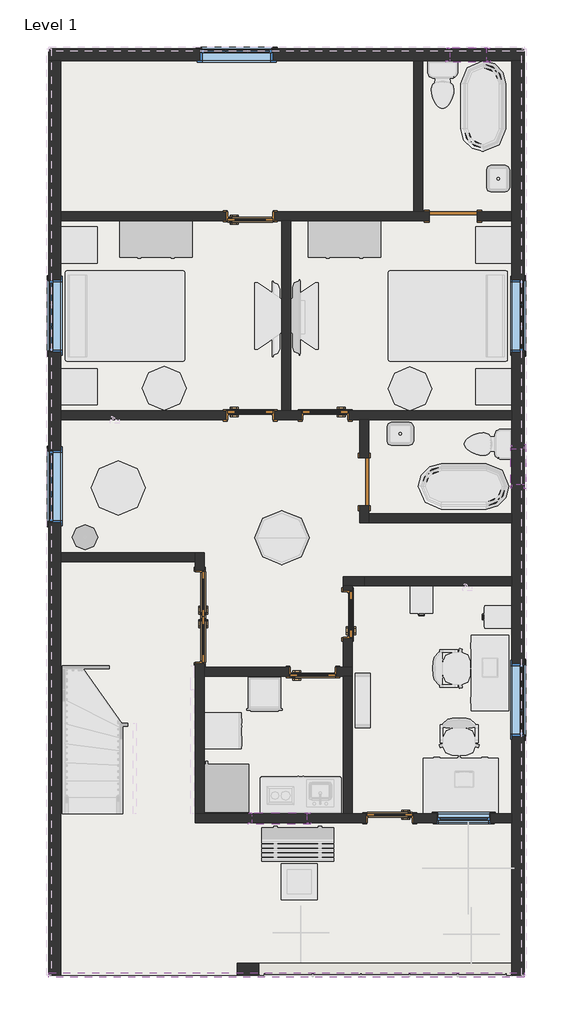
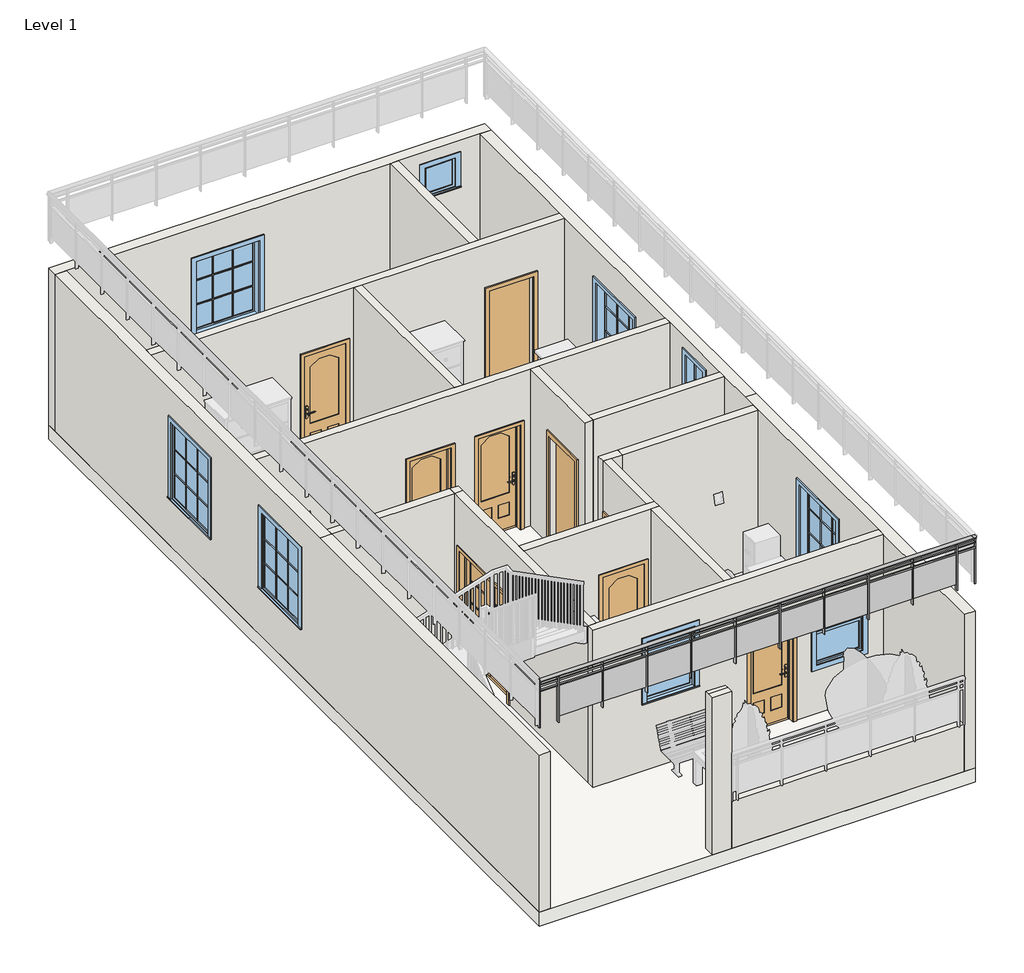
# One storey, part 1 of 4: 19 walls, 9 doors, 9 windows, 1 railing, 1 slab.
"""IFC4 building model written with IfcOpenShell, lengths in millimetres."""

from ifc_helpers import new_model, si_unit, point, frame, origin, origin_with_axes, place, context, project, spatial, polyline, ellipse_curve, trimmed, outline, extrude, faceted_brep, transform, mapped, element, save
from ifc_brep_helpers import plane_surface, extruded_surface, advanced_brep
from components import door_14b9be53, door_4b146b56, door_94998e6c, door_bb092f7c, door_377e7377, window_99fc0ff6, window_d24d93a6, window_e41d21a6

model = new_model("IFC4")

# Units and contexts
model_context = context("Model", 3, world=origin())
ifc_project = project(units=[si_unit("LENGTHUNIT", "METRE", prefix="MILLI")], contexts=[model_context])

# Site, building, storey
site = spatial("IfcSite", under=ifc_project)
building = spatial("IfcBuilding", under=site)
storey = spatial("IfcBuildingStorey", under=building, Name="Level 1", Elevation=0.0)

# Doors
placement = place(None, origin())
door_shape = door_14b9be53(model_context)
element("IfcDoor", 1, ObjectType="30\" x 80\"", at=placement, inside=storey, context=model_context, shape_type="MappedRepresentation", body=[
    mapped(door_shape, transform((-9119.5568901, 3176.746124, 0.0), x_axis=(-1.0, 0.0, 0.0), y_axis=(0.0, -1.0, 0.0), z_axis=(0.0, 0.0, 1.0))),
])
element("IfcDoor", 2, ObjectType="30\" x 80\"", at=placement, inside=storey, context=model_context, shape_type="MappedRepresentation", body=[
    mapped(door_shape, transform((-8532.1818901, 4145.121124, 0.0), x_axis=(0.0, -1.0, 0.0), y_axis=(1.0, 0.0, 0.0), z_axis=(0.0, 0.0, 1.0))),
])
element("IfcDoor", 3, ObjectType="30\" x 80\"", at=placement, inside=storey, context=model_context, shape_type="MappedRepresentation", body=[
    mapped(door_shape, transform((-8910.0068901, 7501.096124, 0.0), x_axis=(1.0, 0.0, 0.0), y_axis=(0.0, 1.0, 0.0), z_axis=(0.0, 0.0, 1.0))),
])
element("IfcDoor", 4, ObjectType="30\" x 80\"", at=placement, inside=storey, context=model_context, shape_type="MappedRepresentation", body=[
    mapped(door_shape, transform((-10173.6568901, 10847.546124, 0.0), x_axis=(-1.0, 0.0, 0.0), y_axis=(0.0, -1.0, 0.0), z_axis=(0.0, 0.0, 1.0))),
])
element("IfcDoor", 5, ObjectType="30\" x 80\"", at=placement, inside=storey, context=model_context, shape_type="MappedRepresentation", body=[
    mapped(door_shape, transform((-7824.1568901, 719.296124, 0.0), x_axis=(1.0, 0.0, 0.0), y_axis=(0.0, 1.0, 0.0), z_axis=(0.0, 0.0, 1.0))),
])
door_2_shape = door_4b146b56(model_context)
element("IfcDoor", 6, ObjectType="30\" x 80\"", at=placement, inside=storey, context=model_context, shape_type="MappedRepresentation", body=[
    mapped(door_2_shape, transform((-10173.6568901, 7501.096124, 0.0), x_axis=(-1.0, 0.0, 0.0), y_axis=(0.0, -1.0, 0.0), z_axis=(0.0, 0.0, 1.0))),
])
door_3_shape = door_94998e6c(model_context)
element("IfcDoor", 7, ObjectType="Door-Exterior-Double-Full Glass-Wood_Clad : 60\" x 80\"", at=placement, inside=storey, context=model_context, shape_type="MappedRepresentation", body=[
    mapped(door_3_shape, transform((-11021.3818901, 4107.021124, 0.0), x_axis=(0.0, -1.0, 0.0), y_axis=(1.0, 0.0, 0.0), z_axis=(0.0, 0.0, 1.0))),
])
door_4_shape = door_bb092f7c(model_context)
element("IfcDoor", 8, ObjectType="Single-Flush : 32\" x 84\"", at=placement, inside=storey, context=model_context, shape_type="MappedRepresentation", body=[
    mapped(door_4_shape, transform((-6757.3568901, 10850.721124, 0.0), x_axis=(-1.0, 0.0, 0.0), y_axis=(0.0, -1.0, 0.0), z_axis=(0.0, 0.0, 1.0))),
])
door_5_shape = door_377e7377(model_context)
element("IfcDoor", 9, ObjectType="Single-Flush : 32\" x 84\"", at=placement, inside=storey, context=model_context, shape_type="MappedRepresentation", body=[
    mapped(door_5_shape, transform((-8255.9568901, 6380.321124, 0.0), x_axis=(0.0, -1.0, 0.0), y_axis=(1.0, 0.0, 0.0), z_axis=(0.0, 0.0, 1.0))),
])

# Railing
element("IfcRailing", 10, ObjectType="Glass Panel - Bottom Fill", at=placement, inside=storey, context=model_context, shape_type="SolidModel", body=[
    advanced_brep(
    [(-13564.5568901, -1887.378876, 4495.8), (-13564.5568901, -1963.578876, 4495.8), (-5563.5568901, -1887.378876, 4495.8), (-5563.5568901, -1963.578876, 4495.8)],
    [
        (0, 1, ellipse_curve(frame((-13564.5568901, -1925.478876, 4495.8), z_axis=(-1.0, 0.0, 0.0), x_axis=(0.0, -1.0, 0.0)), 38.1, 28.575)),
        (1, 0, ellipse_curve(frame((-13564.5568901, -1925.478876, 4495.8), z_axis=(-1.0, 0.0, 0.0), x_axis=(0.0, -1.0, 0.0)), 38.1, 28.575)),
        (2, 3, ellipse_curve(frame((-5563.5568901, -1925.478876, 4495.8), z_axis=(1.0, 0.0, 0.0), x_axis=(0.0, -1.0, 0.0)), 38.1, 28.575)),
        (3, 2, ellipse_curve(frame((-5563.5568901, -1925.478876, 4495.8), z_axis=(1.0, 0.0, 0.0), x_axis=(0.0, -1.0, 0.0)), 38.1, 28.575)),
        (0, 2),
        (3, 1),
    ],
    [
        plane_surface(frame((-13564.5568901, -1925.478876, 4495.8), z_axis=(-1.0, 0.0, 0.0), x_axis=(0.0, 1.0, 0.0))),
        plane_surface(frame((-5563.5568901, -1925.478876, 4495.8), z_axis=(1.0, 0.0, 0.0), x_axis=(0.0, 1.0, 0.0))),
        extruded_surface(trimmed(ellipse_curve(frame((-5563.5568901, -1925.478876, 4495.8), z_axis=(-1.0, 0.0, 0.0), x_axis=(0.0, -1.0, 0.0)), 38.1, 28.575), [point((-5563.5568901, -1887.378876, 4495.8))], [point((-5563.5568901, -1963.578876, 4495.8))], True, "CARTESIAN"), (-8001.000000000001, 0.0, 0.0), 8001.000000000001),
        extruded_surface(trimmed(ellipse_curve(frame((-5563.5568901, -1925.478876, 4495.8), z_axis=(-1.0, 0.0, 0.0), x_axis=(0.0, -1.0, 0.0)), 38.1, 28.575), [point((-5563.5568901, -1963.578876, 4495.8))], [point((-5563.5568901, -1887.378876, 4495.8))], True, "CARTESIAN"), (-8001.000000000001, 0.0, 0.0), 8001.000000000001),
    ],
    [
        (0, [[1, 2]]),
        (1, [[3, 4]]),
        (2, [[-1, 5, -4, 6]]),
        (3, [[-2, -6, -3, -5]]),
    ],
),
    extrude(outline(polyline([(-13564.5568901, -1938.178876), (-13564.5568901, -1912.778876), (-5563.5568901, -1912.778876), (-5563.5568901, -1938.178876), (-13564.5568901, -1938.178876)])), frame((0.0, 0.0, 4381.5), z_axis=(0.0, 0.0, 1.0), x_axis=(1.0, 0.0, 0.0)), (0.0, 0.0, 1.0), 25.4),
    extrude(outline(polyline([(-13564.5568901, -1938.178876), (-13564.5568901, -1912.778876), (-5563.5568901, -1912.778876), (-5563.5568901, -1938.178876), (-13564.5568901, -1938.178876)])), frame((0.0, 0.0, 4279.9), z_axis=(0.0, 0.0, 1.0), x_axis=(1.0, 0.0, 0.0)), (0.0, 0.0, 1.0), 25.4),
    extrude(outline(polyline([(-5912.8068901, -1950.878876), (-5912.8068901, -1900.078876), (-5900.1068901, -1900.078876), (-5900.1068901, -1950.878876), (-5912.8068901, -1950.878876)])), frame((0.0, 0.0, 3581.4), z_axis=(0.0, 0.0, 1.0), x_axis=(1.0, 0.0, 0.0)), (0.0, 0.0, 1.0), 885.6788223),
    extrude(outline(polyline([(-6719.2568901, -1918.943719), (-5906.4568901, -1918.943719), (-5906.4568901, -1925.293719), (-6719.2568901, -1925.293719), (-6719.2568901, -1918.943719)])), frame((0.0, 0.0, 3683.0), z_axis=(0.0, 0.0, 1.0), x_axis=(1.0, 0.0, 0.0)), (0.0, 0.0, 1.0), 596.9),
    extrude(outline(polyline([(-6725.6068901, -1950.878876), (-6725.6068901, -1900.078876), (-6712.9068901, -1900.078876), (-6712.9068901, -1950.878876), (-6725.6068901, -1950.878876)])), frame((0.0, 0.0, 3581.4), z_axis=(0.0, 0.0, 1.0), x_axis=(1.0, 0.0, 0.0)), (0.0, 0.0, 1.0), 885.6788223),
    extrude(outline(polyline([(-7532.0568901, -1918.943719), (-6719.2568901, -1918.943719), (-6719.2568901, -1925.293719), (-7532.0568901, -1925.293719), (-7532.0568901, -1918.943719)])), frame((0.0, 0.0, 3683.0), z_axis=(0.0, 0.0, 1.0), x_axis=(1.0, 0.0, 0.0)), (0.0, 0.0, 1.0), 596.9),
    extrude(outline(polyline([(-7538.4068901, -1950.878876), (-7538.4068901, -1900.078876), (-7525.7068901, -1900.078876), (-7525.7068901, -1950.878876), (-7538.4068901, -1950.878876)])), frame((0.0, 0.0, 3581.4), z_axis=(0.0, 0.0, 1.0), x_axis=(1.0, 0.0, 0.0)), (0.0, 0.0, 1.0), 885.6788223),
    extrude(outline(polyline([(-8344.8568901, -1918.943719), (-7532.0568901, -1918.943719), (-7532.0568901, -1925.293719), (-8344.8568901, -1925.293719), (-8344.8568901, -1918.943719)])), frame((0.0, 0.0, 3683.0), z_axis=(0.0, 0.0, 1.0), x_axis=(1.0, 0.0, 0.0)), (0.0, 0.0, 1.0), 596.9),
    extrude(outline(polyline([(-8351.2068901, -1950.878876), (-8351.2068901, -1900.078876), (-8338.5068901, -1900.078876), (-8338.5068901, -1950.878876), (-8351.2068901, -1950.878876)])), frame((0.0, 0.0, 3581.4), z_axis=(0.0, 0.0, 1.0), x_axis=(1.0, 0.0, 0.0)), (0.0, 0.0, 1.0), 885.6788223),
    extrude(outline(polyline([(-9157.6568901, -1918.943719), (-8344.8568901, -1918.943719), (-8344.8568901, -1925.293719), (-9157.6568901, -1925.293719), (-9157.6568901, -1918.943719)])), frame((0.0, 0.0, 3683.0), z_axis=(0.0, 0.0, 1.0), x_axis=(1.0, 0.0, 0.0)), (0.0, 0.0, 1.0), 596.9),
    extrude(outline(polyline([(-9164.0068901, -1950.878876), (-9164.0068901, -1900.078876), (-9151.3068901, -1900.078876), (-9151.3068901, -1950.878876), (-9164.0068901, -1950.878876)])), frame((0.0, 0.0, 3581.4), z_axis=(0.0, 0.0, 1.0), x_axis=(1.0, 0.0, 0.0)), (0.0, 0.0, 1.0), 885.6788223),
    extrude(outline(polyline([(-9970.4568901, -1918.943719), (-9157.6568901, -1918.943719), (-9157.6568901, -1925.293719), (-9970.4568901, -1925.293719), (-9970.4568901, -1918.943719)])), frame((0.0, 0.0, 3683.0), z_axis=(0.0, 0.0, 1.0), x_axis=(1.0, 0.0, 0.0)), (0.0, 0.0, 1.0), 596.9),
    extrude(outline(polyline([(-9976.8068901, -1950.878876), (-9976.8068901, -1900.078876), (-9964.1068901, -1900.078876), (-9964.1068901, -1950.878876), (-9976.8068901, -1950.878876)])), frame((0.0, 0.0, 3581.4), z_axis=(0.0, 0.0, 1.0), x_axis=(1.0, 0.0, 0.0)), (0.0, 0.0, 1.0), 885.6788223),
    extrude(outline(polyline([(-10783.2568901, -1918.943719), (-9970.4568901, -1918.943719), (-9970.4568901, -1925.293719), (-10783.2568901, -1925.293719), (-10783.2568901, -1918.943719)])), frame((0.0, 0.0, 3683.0), z_axis=(0.0, 0.0, 1.0), x_axis=(1.0, 0.0, 0.0)), (0.0, 0.0, 1.0), 596.9),
    extrude(outline(polyline([(-10789.6068901, -1950.878876), (-10789.6068901, -1900.078876), (-10776.9068901, -1900.078876), (-10776.9068901, -1950.878876), (-10789.6068901, -1950.878876)])), frame((0.0, 0.0, 3581.4), z_axis=(0.0, 0.0, 1.0), x_axis=(1.0, 0.0, 0.0)), (0.0, 0.0, 1.0), 885.6788223),
    extrude(outline(polyline([(-11596.0568901, -1918.943719), (-10783.2568901, -1918.943719), (-10783.2568901, -1925.293719), (-11596.0568901, -1925.293719), (-11596.0568901, -1918.943719)])), frame((0.0, 0.0, 3683.0), z_axis=(0.0, 0.0, 1.0), x_axis=(1.0, 0.0, 0.0)), (0.0, 0.0, 1.0), 596.9),
    extrude(outline(polyline([(-11602.4068901, -1950.878876), (-11602.4068901, -1900.078876), (-11589.7068901, -1900.078876), (-11589.7068901, -1950.878876), (-11602.4068901, -1950.878876)])), frame((0.0, 0.0, 3581.4), z_axis=(0.0, 0.0, 1.0), x_axis=(1.0, 0.0, 0.0)), (0.0, 0.0, 1.0), 885.6788223),
    extrude(outline(polyline([(-12408.8568901, -1918.943719), (-11596.0568901, -1918.943719), (-11596.0568901, -1925.293719), (-12408.8568901, -1925.293719), (-12408.8568901, -1918.943719)])), frame((0.0, 0.0, 3683.0), z_axis=(0.0, 0.0, 1.0), x_axis=(1.0, 0.0, 0.0)), (0.0, 0.0, 1.0), 596.9),
    extrude(outline(polyline([(-12415.2068901, -1950.878876), (-12415.2068901, -1900.078876), (-12402.5068901, -1900.078876), (-12402.5068901, -1950.878876), (-12415.2068901, -1950.878876)])), frame((0.0, 0.0, 3581.4), z_axis=(0.0, 0.0, 1.0), x_axis=(1.0, 0.0, 0.0)), (0.0, 0.0, 1.0), 885.6788223),
    extrude(outline(polyline([(-13221.6568901, -1918.943719), (-12408.8568901, -1918.943719), (-12408.8568901, -1925.293719), (-13221.6568901, -1925.293719), (-13221.6568901, -1918.943719)])), frame((0.0, 0.0, 3683.0), z_axis=(0.0, 0.0, 1.0), x_axis=(1.0, 0.0, 0.0)), (0.0, 0.0, 1.0), 596.9),
    extrude(outline(polyline([(-13228.0068901, -1950.878876), (-13228.0068901, -1900.078876), (-13215.3068901, -1900.078876), (-13215.3068901, -1950.878876), (-13228.0068901, -1950.878876)])), frame((0.0, 0.0, 3581.4), z_axis=(0.0, 0.0, 1.0), x_axis=(1.0, 0.0, 0.0)), (0.0, 0.0, 1.0), 885.6788223),
    extrude(outline(polyline([(-5576.2568901, -1935.003876), (-5576.2568901, -1915.953876), (-5557.2068901, -1915.953876), (-5557.2068901, -1935.003876), (-5576.2568901, -1935.003876)])), frame((0.0, 0.0, 3581.4), z_axis=(0.0, 0.0, 1.0), x_axis=(1.0, 0.0, 0.0)), (0.0, 0.0, 1.0), 885.6788223),
    extrude(outline(polyline([(-13570.9068901, -1935.003876), (-13570.9068901, -1915.953876), (-13551.8568901, -1915.953876), (-13551.8568901, -1935.003876), (-13570.9068901, -1935.003876)])), frame((0.0, 0.0, 3581.4), z_axis=(0.0, 0.0, 1.0), x_axis=(1.0, 0.0, 0.0)), (0.0, 0.0, 1.0), 885.6788223),
])

# Slab
element("IfcSlab", 11, ObjectType="Wood Joist 10\" - Ceramic Tile", at=placement, inside=storey, context=model_context, shape_type="SweptSolid", body=[
    extrude(outline(polyline([(-5563.5568901, 13670.121124), (-5563.5568901, -1925.478876), (-13564.5568901, -1925.478876), (-13564.5568901, 13670.121124), (-5563.5568901, 13670.121124)])), frame((0.0, 0.0, -273.05), z_axis=(0.0, 0.0, 1.0), x_axis=(1.0, 0.0, 0.0)), (0.0, 0.0, 1.0), 273.05),
])

# Walls
element("IfcWall", 12, ObjectType="Generic - 8\"", at=placement, inside=storey, context=model_context, shape_type="Brep", body=[
    faceted_brep([(-13564.5568901, 13466.921124, 0.0), (-13361.3568901, 13466.921124, 0.0), (-7417.7568901, 13466.921124, 0.0), (-7265.3568901, 13466.921124, 0.0), (-5766.7568901, 13466.921124, 0.0), (-5563.5568901, 13466.921124, 0.0), (-5563.5568901, 13466.921124, 3048.0), (-5766.7568901, 13466.921124, 3048.0), (-7265.3568901, 13466.921124, 3048.0), (-7417.7568901, 13466.921124, 3048.0), (-13361.3568901, 13466.921124, 3048.0), (-13564.5568901, 13466.921124, 3048.0), (-9792.6568901, 13466.921124, 2438.4), (-9792.6568901, 13466.921124, 914.4), (-11011.8568901, 13466.921124, 914.4), (-11011.8568901, 13466.921124, 2438.4), (-6808.1568901, 13466.921124, 2768.6), (-6198.5568901, 13466.921124, 2768.6), (-6198.5568901, 13466.921124, 2159.0), (-6808.1568901, 13466.921124, 2159.0), (-13564.5568901, 13670.121124, 0.0), (-13564.5568901, 13670.121124, 3048.0), (-5563.5568901, 13670.121124, 3048.0), (-5563.5568901, 13670.121124, 0.0), (-9792.6568901, 13670.121124, 2438.4), (-11011.8568901, 13670.121124, 2438.4), (-11011.8568901, 13670.121124, 914.4), (-9792.6568901, 13670.121124, 914.4), (-6808.1568901, 13670.121124, 2768.6), (-6808.1568901, 13670.121124, 2159.0), (-6198.5568901, 13670.121124, 2159.0), (-6198.5568901, 13670.121124, 2768.6)], [[[0, 1, 2, 3, 4, 5, 6, 7, 8, 9, 10, 11], [12, 13, 14, 15], [16, 17, 18, 19]], [[20, 21, 22, 23], [24, 25, 26, 27], [28, 29, 30, 31]], [[5, 4, 3, 2, 1, 0, 20, 23]], [[6, 5, 23, 22]], [[0, 11, 21, 20]], [[11, 10, 9, 8, 7, 6, 22, 21]], [[13, 12, 24, 27]], [[14, 13, 27, 26]], [[15, 14, 26, 25]], [[12, 15, 25, 24]], [[29, 28, 16, 19]], [[30, 29, 19, 18]], [[31, 30, 18, 17]], [[28, 31, 17, 16]]]),
])
element("IfcWall", 13, ObjectType="Generic - 8\"", at=placement, inside=storey, context=model_context, shape_type="Brep", body=[
    faceted_brep([(-5766.7568901, 13466.921124, 0.0), (-5766.7568901, 10926.921124, 0.0), (-5766.7568901, 10774.521124, 0.0), (-5766.7568901, 7574.121124, 0.0), (-5766.7568901, 7421.721124, 0.0), (-5766.7568901, 5846.921124, 0.0), (-5766.7568901, 5694.521124, 0.0), (-5766.7568901, 4780.121124, 0.0), (-5766.7568901, 4627.721124, 0.0), (-5766.7568901, 792.321124, 0.0), (-5766.7568901, 639.921124, 0.0), (-5766.7568901, -1722.278876, 0.0), (-5766.7568901, -1925.478876, 0.0), (-5766.7568901, -1925.478876, 914.4), (-5766.7568901, -1925.478876, 3048.0), (-5766.7568901, 639.921124, 3048.0), (-5766.7568901, 792.321124, 3048.0), (-5766.7568901, 4627.721124, 3048.0), (-5766.7568901, 4780.121124, 3048.0), (-5766.7568901, 5034.121124, 3048.0), (-5766.7568901, 5694.521124, 3048.0), (-5766.7568901, 5846.921124, 3048.0), (-5766.7568901, 7421.721124, 3048.0), (-5766.7568901, 7574.121124, 3048.0), (-5766.7568901, 10774.521124, 3048.0), (-5766.7568901, 10926.921124, 3048.0), (-5766.7568901, 13466.921124, 3048.0), (-5766.7568901, 2100.421124, 2438.4), (-5766.7568901, 2100.421124, 914.4), (-5766.7568901, 3319.621124, 914.4), (-5766.7568901, 3319.621124, 2438.4), (-5766.7568901, 8564.721124, 2438.4), (-5766.7568901, 8564.721124, 914.4), (-5766.7568901, 9783.921124, 914.4), (-5766.7568901, 9783.921124, 2438.4), (-5766.7568901, 6329.521124, 2768.6), (-5766.7568901, 6329.521124, 2159.0), (-5766.7568901, 6939.121124, 2159.0), (-5766.7568901, 6939.121124, 2768.6), (-5563.5568901, 13466.921124, 0.0), (-5563.5568901, 13466.921124, 3048.0), (-5563.5568901, 5034.121124, 3048.0), (-5563.5568901, -1925.478876, 3048.0), (-5563.5568901, -1925.478876, 0.0), (-5563.5568901, 2100.421124, 2438.4), (-5563.5568901, 3319.621124, 2438.4), (-5563.5568901, 3319.621124, 914.4), (-5563.5568901, 2100.421124, 914.4), (-5563.5568901, 8564.721124, 2438.4), (-5563.5568901, 9783.921124, 2438.4), (-5563.5568901, 9783.921124, 914.4), (-5563.5568901, 8564.721124, 914.4), (-5563.5568901, 6329.521124, 2768.6), (-5563.5568901, 6939.121124, 2768.6), (-5563.5568901, 6939.121124, 2159.0), (-5563.5568901, 6329.521124, 2159.0)], [[[0, 1, 2, 3, 4, 5, 6, 7, 8, 9, 10, 11, 12, 13, 14, 15, 16, 17, 18, 19, 20, 21, 22, 23, 24, 25, 26], [27, 28, 29, 30], [31, 32, 33, 34], [35, 36, 37, 38]], [[39, 40, 41, 42, 43], [44, 45, 46, 47], [48, 49, 50, 51], [52, 53, 54, 55]], [[12, 11, 10, 9, 8, 7, 6, 5, 4, 3, 2, 1, 0, 39, 43]], [[0, 26, 40, 39]], [[14, 13, 12, 43, 42]], [[19, 18, 17, 16, 15, 14, 42, 41]], [[26, 25, 24, 23, 22, 21, 20, 19, 41, 40]], [[28, 27, 44, 47]], [[29, 28, 47, 46]], [[30, 29, 46, 45]], [[27, 30, 45, 44]], [[32, 31, 48, 51]], [[33, 32, 51, 50]], [[34, 33, 50, 49]], [[31, 34, 49, 48]], [[36, 35, 52, 55]], [[37, 36, 55, 54]], [[38, 37, 54, 53]], [[35, 38, 53, 52]]]),
])
element("IfcWall", 14, ObjectType="Generic - 8\"", at=placement, inside=storey, context=model_context, shape_type="SweptSolid", body=[
    extrude(outline(polyline([(-10033.9568901, -1722.278876), (-5766.7568901, -1722.278876), (-5766.7568901, -1925.478876), (-10033.9568901, -1925.478876), (-10033.9568901, -1722.278876)])), origin_with_axes(), (0.0, 0.0, 1.0), 914.4),
])
element("IfcWall", 15, ObjectType="Generic - 8\"", at=placement, inside=storey, context=model_context, shape_type="Brep", body=[
    faceted_brep([(-13361.3568901, -1925.478876, 0.0), (-13361.3568901, 5034.121124, 0.0), (-13361.3568901, 5186.521124, 0.0), (-13361.3568901, 7421.721124, 0.0), (-13361.3568901, 7574.121124, 0.0), (-13361.3568901, 10774.521124, 0.0), (-13361.3568901, 10926.921124, 0.0), (-13361.3568901, 13466.921124, 0.0), (-13361.3568901, 13466.921124, 3048.0), (-13361.3568901, 10926.921124, 3048.0), (-13361.3568901, 10774.521124, 3048.0), (-13361.3568901, 7574.121124, 3048.0), (-13361.3568901, 7421.721124, 3048.0), (-13361.3568901, 5186.521124, 3048.0), (-13361.3568901, 5034.121124, 3048.0), (-13361.3568901, -1925.478876, 3048.0), (-13361.3568901, 9783.921124, 2438.4), (-13361.3568901, 9783.921124, 914.4), (-13361.3568901, 8564.721124, 914.4), (-13361.3568901, 8564.721124, 2438.4), (-13361.3568901, 6913.721124, 2438.4), (-13361.3568901, 6913.721124, 914.4), (-13361.3568901, 5694.521124, 914.4), (-13361.3568901, 5694.521124, 2438.4), (-13564.5568901, -1925.478876, 0.0), (-13564.5568901, -1925.478876, 3048.0), (-13564.5568901, 5034.121124, 3048.0), (-13564.5568901, 13466.921124, 3048.0), (-13564.5568901, 13466.921124, 0.0), (-13564.5568901, 9783.921124, 2438.4), (-13564.5568901, 8564.721124, 2438.4), (-13564.5568901, 8564.721124, 914.4), (-13564.5568901, 9783.921124, 914.4), (-13564.5568901, 6913.721124, 2438.4), (-13564.5568901, 5694.521124, 2438.4), (-13564.5568901, 5694.521124, 914.4), (-13564.5568901, 6913.721124, 914.4)], [[[0, 1, 2, 3, 4, 5, 6, 7, 8, 9, 10, 11, 12, 13, 14, 15], [16, 17, 18, 19], [20, 21, 22, 23]], [[24, 25, 26, 27, 28], [29, 30, 31, 32], [33, 34, 35, 36]], [[7, 6, 5, 4, 3, 2, 1, 0, 24, 28]], [[0, 15, 25, 24]], [[8, 7, 28, 27]], [[15, 14, 26, 25]], [[14, 13, 12, 11, 10, 9, 8, 27, 26]], [[17, 16, 29, 32]], [[18, 17, 32, 31]], [[19, 18, 31, 30]], [[16, 19, 30, 29]], [[21, 20, 33, 36]], [[22, 21, 36, 35]], [[23, 22, 35, 34]], [[20, 23, 34, 33]]]),
])
element("IfcWall", 16, ObjectType="Generic - 8\"", at=placement, inside=storey, context=model_context, shape_type="Brep", body=[
    faceted_brep([(-10033.9568901, -1722.278876, 0.0), (-10389.5568901, -1722.278876, 0.0), (-10389.5568901, -1722.278876, 3048.0), (-10033.9568901, -1722.278876, 3048.0), (-10033.9568901, -1722.278876, 914.4), (-10033.9568901, -1925.478876, 0.0), (-10033.9568901, -1925.478876, 914.4), (-10033.9568901, -1925.478876, 3048.0), (-10389.5568901, -1925.478876, 3048.0), (-10389.5568901, -1925.478876, 0.0), (-10389.5568901, -1798.478876, 3048.0), (-10033.9568901, -1798.478876, 3048.0)], [[[0, 1, 2, 3, 4]], [[5, 6, 7, 8, 9]], [[1, 0, 5, 9]], [[2, 1, 9, 8, 10]], [[0, 4, 3, 11, 7, 6, 5]], [[3, 2, 10, 11]], [[10, 8, 7, 11]]]),
])
element("IfcWall", 17, ObjectType="INNER WALL", at=placement, inside=storey, context=model_context, shape_type="Brep", body=[
    faceted_brep([(-5766.7568901, 10774.521124, 0.0), (-5766.7568901, 10774.521124, 3048.0), (-9487.8568901, 10774.521124, 3048.0), (-9640.2568901, 10774.521124, 3048.0), (-13361.3568901, 10774.521124, 3048.0), (-13361.3568901, 10774.521124, 0.0), (-10580.0568901, 10774.521124, 0.0), (-10580.0568901, 10774.521124, 2057.4), (-9767.2568901, 10774.521124, 2057.4), (-9767.2568901, 10774.521124, 0.0), (-9640.2568901, 10774.521124, 0.0), (-9487.8568901, 10774.521124, 0.0), (-7163.7568901, 10774.521124, 0.0), (-7163.7568901, 10774.521124, 2133.6), (-6350.9568901, 10774.521124, 2133.6), (-6350.9568901, 10774.521124, 0.0), (-5766.7568901, 10926.921124, 3048.0), (-5766.7568901, 10926.921124, 0.0), (-6350.9568901, 10926.921124, 0.0), (-6350.9568901, 10926.921124, 2133.6), (-7163.7568901, 10926.921124, 2133.6), (-7163.7568901, 10926.921124, 0.0), (-7265.3568901, 10926.921124, 0.0), (-7417.7568901, 10926.921124, 0.0), (-9767.2568901, 10926.921124, 0.0), (-9767.2568901, 10926.921124, 2057.4), (-10580.0568901, 10926.921124, 2057.4), (-10580.0568901, 10926.921124, 0.0), (-13361.3568901, 10926.921124, 0.0), (-13361.3568901, 10926.921124, 3048.0), (-7417.7568901, 10926.921124, 3048.0), (-7265.3568901, 10926.921124, 3048.0)], [[[0, 1, 2, 3, 4, 5, 6, 7, 8, 9, 10, 11, 12, 13, 14, 15]], [[16, 17, 18, 19, 20, 21, 22, 23, 24, 25, 26, 27, 28, 29, 30, 31]], [[5, 28, 27, 6]], [[17, 0, 15, 18]], [[21, 12, 11, 10, 9, 24, 23, 22]], [[1, 0, 17, 16]], [[5, 4, 29, 28]], [[13, 12, 21, 20]], [[14, 13, 20, 19]], [[15, 14, 19, 18]], [[26, 7, 6, 27]], [[7, 26, 25, 8]], [[8, 25, 24, 9]], [[4, 3, 2, 1, 16, 31, 30, 29]]]),
])
element("IfcWall", 18, ObjectType="INNER WALL", at=placement, inside=storey, context=model_context, shape_type="Brep", body=[
    faceted_brep([(-5766.7568901, 7421.721124, 0.0), (-5766.7568901, 7421.721124, 3048.0), (-8179.7568901, 7421.721124, 3048.0), (-8332.1568901, 7421.721124, 3048.0), (-13361.3568901, 7421.721124, 3048.0), (-13361.3568901, 7421.721124, 0.0), (-10580.0568901, 7421.721124, 0.0), (-10580.0568901, 7421.721124, 2057.4), (-9767.2568901, 7421.721124, 2057.4), (-9767.2568901, 7421.721124, 0.0), (-9316.4068901, 7421.721124, 0.0), (-9316.4068901, 7421.721124, 2057.4), (-8503.6068901, 7421.721124, 2057.4), (-8503.6068901, 7421.721124, 0.0), (-8332.1568901, 7421.721124, 0.0), (-8179.7568901, 7421.721124, 0.0), (-5766.7568901, 7574.121124, 3048.0), (-5766.7568901, 7574.121124, 0.0), (-8503.6068901, 7574.121124, 0.0), (-8503.6068901, 7574.121124, 2057.4), (-9316.4068901, 7574.121124, 2057.4), (-9316.4068901, 7574.121124, 0.0), (-9487.8568901, 7574.121124, 0.0), (-9640.2568901, 7574.121124, 0.0), (-9767.2568901, 7574.121124, 0.0), (-9767.2568901, 7574.121124, 2057.4), (-10580.0568901, 7574.121124, 2057.4), (-10580.0568901, 7574.121124, 0.0), (-13361.3568901, 7574.121124, 0.0), (-13361.3568901, 7574.121124, 3048.0), (-9640.2568901, 7574.121124, 3048.0), (-9487.8568901, 7574.121124, 3048.0)], [[[0, 1, 2, 3, 4, 5, 6, 7, 8, 9, 10, 11, 12, 13, 14, 15]], [[16, 17, 18, 19, 20, 21, 22, 23, 24, 25, 26, 27, 28, 29, 30, 31]], [[5, 28, 27, 6]], [[17, 0, 15, 14, 13, 18]], [[21, 10, 9, 24, 23, 22]], [[1, 0, 17, 16]], [[5, 4, 29, 28]], [[12, 19, 18, 13]], [[19, 12, 11, 20]], [[20, 11, 10, 21]], [[26, 7, 6, 27]], [[7, 26, 25, 8]], [[8, 25, 24, 9]], [[4, 3, 2, 1, 16, 31, 30, 29]]]),
])
element("IfcWall", 19, ObjectType="INNER WALL", at=placement, inside=storey, context=model_context, shape_type="Brep", body=[
    faceted_brep([(-5766.7568901, 792.321124, 3048.0), (-5766.7568901, 792.321124, 0.0), (-7417.7568901, 792.321124, 0.0), (-7417.7568901, 792.321124, 2057.4), (-8230.5568901, 792.321124, 2057.4), (-8230.5568901, 792.321124, 0.0), (-8459.1568901, 792.321124, 0.0), (-8611.5568901, 792.321124, 0.0), (-10948.3568901, 792.321124, 0.0), (-11100.7568901, 792.321124, 0.0), (-11100.7568901, 792.321124, 3048.0), (-10948.3568901, 792.321124, 3048.0), (-8611.5568901, 792.321124, 3048.0), (-8459.1568901, 792.321124, 3048.0), (-10135.5568901, 792.321124, 2514.6), (-10135.5568901, 792.321124, 1295.4), (-9221.1568901, 792.321124, 1295.4), (-9221.1568901, 792.321124, 2514.6), (-6122.3568901, 792.321124, 2133.6), (-7036.7568901, 792.321124, 2133.6), (-7036.7568901, 792.321124, 914.4), (-6122.3568901, 792.321124, 914.4), (-5766.7568901, 639.921124, 0.0), (-5766.7568901, 639.921124, 3048.0), (-11100.7568901, 639.921124, 3048.0), (-11100.7568901, 639.921124, 0.0), (-8230.5568901, 639.921124, 0.0), (-8230.5568901, 639.921124, 2057.4), (-7417.7568901, 639.921124, 2057.4), (-7417.7568901, 639.921124, 0.0), (-10135.5568901, 639.921124, 2514.6), (-9221.1568901, 639.921124, 2514.6), (-9221.1568901, 639.921124, 1295.4), (-10135.5568901, 639.921124, 1295.4), (-6122.3568901, 639.921124, 2133.6), (-6122.3568901, 639.921124, 914.4), (-7036.7568901, 639.921124, 914.4), (-7036.7568901, 639.921124, 2133.6)], [[[0, 1, 2, 3, 4, 5, 6, 7, 8, 9, 10, 11, 12, 13], [14, 15, 16, 17], [18, 19, 20, 21]], [[22, 23, 24, 25, 26, 27, 28, 29], [30, 31, 32, 33], [34, 35, 36, 37]], [[1, 22, 29, 2]], [[25, 9, 8, 7, 6, 5, 26]], [[1, 0, 23, 22]], [[10, 9, 25, 24]], [[0, 13, 12, 11, 10, 24, 23]], [[15, 14, 30, 33]], [[16, 15, 33, 32]], [[17, 16, 32, 31]], [[14, 17, 31, 30]], [[35, 34, 18, 21]], [[36, 35, 21, 20]], [[37, 36, 20, 19]], [[34, 37, 19, 18]], [[28, 3, 2, 29]], [[3, 28, 27, 4]], [[4, 27, 26, 5]]]),
])
element("IfcWall", 20, ObjectType="INNER WALL", at=placement, inside=storey, context=model_context, shape_type="SweptSolid", body=[
    extrude(outline(polyline([(-8459.1568901, 3103.721124), (-8459.1568901, 792.321124), (-8611.5568901, 792.321124), (-8611.5568901, 3103.721124), (-8459.1568901, 3103.721124)])), origin_with_axes(), (0.0, 0.0, 1.0), 3048.0),
])
element("IfcWall", 21, ObjectType="INNER WALL", at=placement, inside=storey, context=model_context, shape_type="Brep", body=[
    faceted_brep([(-10948.3568901, 5186.521124, 0.0), (-10948.3568901, 5186.521124, 3048.0), (-10948.3568901, 5034.121124, 3048.0), (-10948.3568901, 3256.121124, 3048.0), (-10948.3568901, 3103.721124, 3048.0), (-10948.3568901, 792.321124, 3048.0), (-10948.3568901, 792.321124, 0.0), (-10948.3568901, 3103.721124, 0.0), (-10948.3568901, 3256.121124, 0.0), (-10948.3568901, 3319.621124, 0.0), (-10948.3568901, 3319.621124, 2057.4), (-10948.3568901, 4894.421124, 2057.4), (-10948.3568901, 4894.421124, 0.0), (-11100.7568901, 5186.521124, 3048.0), (-11100.7568901, 5186.521124, 0.0), (-11100.7568901, 5034.121124, 0.0), (-11100.7568901, 4894.421124, 0.0), (-11100.7568901, 4894.421124, 2057.4), (-11100.7568901, 3319.621124, 2057.4), (-11100.7568901, 3319.621124, 0.0), (-11100.7568901, 792.321124, 0.0), (-11100.7568901, 792.321124, 3048.0), (-11100.7568901, 5034.121124, 3048.0)], [[[0, 1, 2, 3, 4, 5, 6, 7, 8, 9, 10, 11, 12]], [[13, 14, 15, 16, 17, 18, 19, 20, 21, 22]], [[14, 0, 12, 16, 15]], [[6, 20, 19, 9, 8, 7]], [[1, 0, 14, 13]], [[6, 5, 21, 20]], [[18, 10, 9, 19]], [[10, 18, 17, 11]], [[11, 17, 16, 12]], [[21, 5, 4, 3, 2, 22]], [[2, 1, 13, 22]]]),
])
element("IfcWall", 22, ObjectType="INNER WALL", at=placement, inside=storey, context=model_context, shape_type="SweptSolid", body=[
    extrude(outline(polyline([(-13361.3568901, 5186.521124), (-11100.7568901, 5186.521124), (-11100.7568901, 5034.121124), (-13361.3568901, 5034.121124), (-13361.3568901, 5186.521124)])), origin_with_axes(), (0.0, 0.0, 1.0), 3048.0),
])
element("IfcWall", 23, ObjectType="INNER WALL", at=placement, inside=storey, context=model_context, shape_type="Brep", body=[
    faceted_brep([(-10948.3568901, 3103.721124, 3048.0), (-10948.3568901, 3103.721124, 0.0), (-9525.9568901, 3103.721124, 0.0), (-9525.9568901, 3103.721124, 2057.4), (-8713.1568901, 3103.721124, 2057.4), (-8713.1568901, 3103.721124, 0.0), (-8611.5568901, 3103.721124, 0.0), (-8459.1568901, 3103.721124, 0.0), (-8459.1568901, 3103.721124, 3048.0), (-8611.5568901, 3103.721124, 3048.0), (-10948.3568901, 3256.121124, 0.0), (-10948.3568901, 3256.121124, 3048.0), (-8611.5568901, 3256.121124, 3048.0), (-8459.1568901, 3256.121124, 3048.0), (-8459.1568901, 3256.121124, 0.0), (-8611.5568901, 3256.121124, 0.0), (-8713.1568901, 3256.121124, 0.0), (-8713.1568901, 3256.121124, 2057.4), (-9525.9568901, 3256.121124, 2057.4), (-9525.9568901, 3256.121124, 0.0)], [[[0, 1, 2, 3, 4, 5, 6, 7, 8, 9]], [[10, 11, 12, 13, 14, 15, 16, 17, 18, 19]], [[1, 10, 19, 2]], [[14, 7, 6, 5, 16, 15]], [[1, 0, 11, 10]], [[8, 7, 14, 13]], [[18, 3, 2, 19]], [[3, 18, 17, 4]], [[4, 17, 16, 5]], [[0, 9, 8, 13, 12, 11]]]),
])
element("IfcWall", 24, ObjectType="INNER WALL", at=placement, inside=storey, context=model_context, shape_type="SweptSolid", body=[
    extrude(outline(polyline([(-8255.9568901, 4780.121124), (-5766.7568901, 4780.121124), (-5766.7568901, 4627.721124), (-8255.9568901, 4627.721124), (-8255.9568901, 4780.121124)])), origin_with_axes(), (0.0, 0.0, 1.0), 3048.0),
])
element("IfcWall", 25, ObjectType="INNER WALL", at=placement, inside=storey, context=model_context, shape_type="SweptSolid", body=[
    extrude(outline(polyline([(-8179.7568901, 5846.921124), (-5766.7568901, 5846.921124), (-5766.7568901, 5694.521124), (-8179.7568901, 5694.521124), (-8179.7568901, 5846.921124)])), origin_with_axes(), (0.0, 0.0, 1.0), 3048.0),
])
element("IfcWall", 26, ObjectType="INNER WALL", at=placement, inside=storey, context=model_context, shape_type="SweptSolid", body=[
    extrude(outline(polyline([(-9487.8568901, 10774.521124), (-9487.8568901, 7574.121124), (-9640.2568901, 7574.121124), (-9640.2568901, 10774.521124), (-9487.8568901, 10774.521124)])), origin_with_axes(), (0.0, 0.0, 1.0), 3048.0),
])
element("IfcWall", 27, ObjectType="INNER WALL", at=placement, inside=storey, context=model_context, shape_type="SweptSolid", body=[
    extrude(outline(polyline([(-7265.3568901, 13466.921124), (-7265.3568901, 10926.921124), (-7417.7568901, 10926.921124), (-7417.7568901, 13466.921124), (-7265.3568901, 13466.921124)])), origin_with_axes(), (0.0, 0.0, 1.0), 3048.0),
])
element("IfcWall", 28, ObjectType="INNER WALL", at=placement, inside=storey, context=model_context, shape_type="Brep", body=[
    faceted_brep([(-8179.7568901, 5694.521124, 0.0), (-8179.7568901, 5846.921124, 0.0), (-8179.7568901, 5973.921124, 0.0), (-8179.7568901, 5973.921124, 2133.6), (-8179.7568901, 6786.721124, 2133.6), (-8179.7568901, 6786.721124, 0.0), (-8179.7568901, 7421.721124, 0.0), (-8179.7568901, 7421.721124, 3048.0), (-8179.7568901, 5846.921124, 3048.0), (-8179.7568901, 5694.521124, 3048.0), (-8332.1568901, 5973.921124, 2133.6), (-8332.1568901, 5973.921124, 0.0), (-8332.1568901, 5694.521124, 0.0), (-8332.1568901, 5694.521124, 3048.0), (-8332.1568901, 7421.721124, 3048.0), (-8332.1568901, 7421.721124, 0.0), (-8332.1568901, 6786.721124, 0.0), (-8332.1568901, 6786.721124, 2133.6)], [[[0, 1, 2, 3, 4, 5, 6, 7, 8, 9]], [[10, 11, 12, 13, 14, 15, 16, 17]], [[16, 15, 6, 5]], [[12, 11, 2, 1, 0]], [[7, 6, 15, 14]], [[3, 2, 11, 10]], [[4, 3, 10, 17]], [[5, 4, 17, 16]], [[0, 9, 13, 12]], [[9, 8, 7, 14, 13]]]),
])
element("IfcWall", 29, ObjectType="INNER WALL", at=placement, inside=storey, context=model_context, shape_type="SweptSolid", body=[
    extrude(outline(polyline([(3256.121124, 0.0), (3256.121124, 3048.0), (4627.721124, 3048.0), (4627.721124, 0.0), (4551.521124, 0.0), (4551.521124, 2057.4), (3738.721124, 2057.4), (3738.721124, 0.0), (3256.121124, 0.0)])), frame((-8611.5568901, 0.0, 0.0), z_axis=(1.0, 0.0, 0.0), x_axis=(0.0, 1.0, 0.0)), (0.0, 0.0, 1.0), 152.4),
])
element("IfcWall", 30, ObjectType="INNER WALL", at=placement, inside=storey, context=model_context, shape_type="Brep", body=[
    faceted_brep([(-8255.9568901, 4780.121124, 0.0), (-8611.5568901, 4780.121124, 0.0), (-8611.5568901, 4780.121124, 3048.0), (-8255.9568901, 4780.121124, 3048.0), (-8255.9568901, 4627.721124, 0.0), (-8255.9568901, 4627.721124, 3048.0), (-8459.1568901, 4627.721124, 3048.0), (-8611.5568901, 4627.721124, 3048.0), (-8611.5568901, 4627.721124, 0.0), (-8459.1568901, 4627.721124, 0.0)], [[[0, 1, 2, 3]], [[4, 5, 6, 7, 8, 9]], [[1, 0, 4, 9, 8]], [[0, 3, 5, 4]], [[2, 1, 8, 7]], [[3, 2, 7, 6, 5]]]),
])

# Windows
window_shape = window_99fc0ff6(model_context)
element("IfcWindow", 31, ObjectType="Casement 3x3 with Trim : 48\" x 60\"", at=placement, inside=storey, context=model_context, shape_type="MappedRepresentation", body=[
    mapped(window_shape, transform((-5665.1568901, 2710.021124, 609.6), x_axis=(0.0, -1.0, 0.0), y_axis=(1.0, 0.0, 0.0), z_axis=(0.0, 0.0, 1.0))),
])
element("IfcWindow", 32, ObjectType="Casement 3x3 with Trim : 48\" x 60\"", at=placement, inside=storey, context=model_context, shape_type="MappedRepresentation", body=[
    mapped(window_shape, transform((-5665.1568901, 9174.321124, 609.6), x_axis=(0.0, -1.0, 0.0), y_axis=(1.0, 0.0, 0.0), z_axis=(0.0, 0.0, 1.0))),
])
element("IfcWindow", 33, ObjectType="Casement 3x3 with Trim : 48\" x 60\"", at=placement, inside=storey, context=model_context, shape_type="MappedRepresentation", body=[
    mapped(window_shape, transform((-10402.2568901, 13568.521124, 609.6), x_axis=(1.0, 0.0, 0.0), y_axis=(0.0, 1.0, 0.0), z_axis=(0.0, 0.0, 1.0))),
])
element("IfcWindow", 34, ObjectType="Casement 3x3 with Trim : 48\" x 60\"", at=placement, inside=storey, context=model_context, shape_type="MappedRepresentation", body=[
    mapped(window_shape, transform((-13462.9568901, 9174.321124, 609.6), x_axis=(0.0, 1.0, 0.0), y_axis=(-1.0, 0.0, 0.0), z_axis=(0.0, 0.0, 1.0))),
])
element("IfcWindow", 35, ObjectType="Casement 3x3 with Trim : 48\" x 60\"", at=placement, inside=storey, context=model_context, shape_type="MappedRepresentation", body=[
    mapped(window_shape, transform((-13462.9568901, 6304.121124, 609.6), x_axis=(0.0, 1.0, 0.0), y_axis=(-1.0, 0.0, 0.0), z_axis=(0.0, 0.0, 1.0))),
])
window_2_shape = window_d24d93a6(model_context)
element("IfcWindow", 36, ObjectType="Double Hung with Trim : 36\" x 48\"", at=placement, inside=storey, context=model_context, shape_type="MappedRepresentation", body=[
    mapped(window_2_shape, transform((-9678.3568901, 716.121124, 381.0), x_axis=(-1.0, 0.0, 0.0), y_axis=(0.0, -1.0, 0.0), z_axis=(0.0, 0.0, 1.0))),
])
element("IfcWindow", 37, ObjectType="Double Hung with Trim : 36\" x 48\"", at=placement, inside=storey, context=model_context, shape_type="MappedRepresentation", body=[
    mapped(window_2_shape, transform((-6579.5568901, 716.121124, 0.0), x_axis=(1.0, 0.0, 0.0), y_axis=(0.0, 1.0, 0.0), z_axis=(0.0, 0.0, 1.0))),
])
window_3_shape = window_e41d21a6(model_context)
element("IfcWindow", 38, ObjectType="Transom with Trim : 24\" x 24\"", at=placement, inside=storey, context=model_context, shape_type="MappedRepresentation", body=[
    mapped(window_3_shape, transform((-5665.1568901, 6596.221124, 0.0), x_axis=(0.0, -1.0, 0.0), y_axis=(1.0, 0.0, 0.0), z_axis=(0.0, 0.0, 1.0))),
])
element("IfcWindow", 39, ObjectType="Transom with Trim : 24\" x 24\"", at=placement, inside=storey, context=model_context, shape_type="MappedRepresentation", body=[
    mapped(window_3_shape, transform((-6541.4568901, 13568.521124, 0.0), x_axis=(-1.0, 0.0, 0.0), y_axis=(0.0, -1.0, 0.0), z_axis=(0.0, 0.0, 1.0))),
])

save(model, "model.ifc")

# Revit data of these elements
# Type "30\" x 80\""
#   Type Mark = "9"
#   Assembly Code = "B2030100"
#   Analytic Construction = "French door, wood frame with single glass"
#   Threshold Offset [instance default] = 0' - 0 1/2"
#   Thickness = 0' - 1 3/8"
#   Thermal Resistance (R) = 1.0696 (h·ft²·°F)/BTU
#   Swing Angle [instance default] = 90.00°
#   Stiles = 0' - 4 3/4"
#   Rough Width = 2' - 8"
#   Rough Height = 6' - 9"
#   Radius = 1' - 1.00625"
#   Lock Rail = 0' - 7 1/8"
#   Height = 6' - 8"
#   Width = 2' - 6"
#   Heat Transfer Coefficient (U) = 0.9350 BTU/(h·ft²·°F)
#   Door Offset [instance default] = 0' - 0"
#   Bottom Rail = 0' - 9 1/2"
#   Threshold [instance default] = yes
#   Function = 1
#   Exterior Trim [instance default] = yes
#   Trim Material = Cherry
#   Threshold Material = Cherry
#   Panel Material = Cherry
#   Glazing = Glass
#   Frame Material = Cherry
#   Door Handle Material = Aluminum
#   Visual Light Transmittance = 0
#   Solar Heat Gain Coefficient = 0
#   Wall Closure = (empty or 0)
#   Construction Type = (empty or 0)
# Type "Door-Exterior-Double-Full Glass-Wood_Clad : 60\" x 80\""
#   Type Mark = "8"
#   Assembly Code = "B2030100"
#   Analytic Construction = "French door, wood frame with double glass"
#   Top Rail = 0' - 4 11/16"
#   Threshold Offset [instance default] = 0' - 0 1/2"
#   Thickness = 0' - 1 3/8"
#   Thermal Resistance (R) = 1.9158 (h·ft²·°F)/BTU
#   Swing Angle [instance default] = 90.00°
#   Stiles = 0' - 4 3/4"
#   Rough Width = 5' - 2"
#   Rough Height = 6' - 9"
#   Panel Width = 2' - 6"
#   Door Offset [instance default] = 0' - 0"
#   Height = 6' - 8"
#   Width = 5' - 0"
#   Heat Transfer Coefficient (U) = 0.5220 BTU/(h·ft²·°F)
#   Bottom Rail = 0' - 9 1/8"
#   Exterior Trim [instance default] = yes
#   Threshold [instance default] = yes
#   Show Grill [instance default] = yes
#   Function = 1
#   Trim Material = Cherry
#   Threshold Material = Cherry
#   Panel Material = Cherry
#   Glazing = Glass
#   Frame Material = Cherry
#   Door Handle Material = Aluminum
#   Visual Light Transmittance = 0
#   Solar Heat Gain Coefficient = 0
#   Wall Closure = (empty or 0)
#   Construction Type = (empty or 0)
# Type "Single-Flush : 32\" x 84\""
#   Type Mark = "3"
#   Construction Type Id = "MDOOR"
#   Assembly Code = "C1020"
#   Analytic Construction = "Metal"
#   Thickness = 0' - 2"
#   Heat Transfer Coefficient (U) = 0.651978 BTU/(h·ft²·°F)
#   Height = 7' - 0"
#   Trim Projection Ext = 0' - 1"
#   Trim Projection Int = 0' - 1"
#   Trim Width = 0' - 3"
#   Width = 2' - 8"
#   Define Thermal Properties by = 1
#   Door Material = Door - Panel
#   Frame Material = Door - Frame
#   Visual Light Transmittance = 0
#   Solar Heat Gain Coefficient = 0
#   Function = (empty or 0)
#   Wall Closure = (empty or 0)
# Type "Glass Panel - Bottom Fill"
#   Assembly Code = "C2010400"
#   built-in parameter 1008612 = 0.0416667 (stored number, unit not read)
#   built-in parameter 1008611 = 0.0416667 (stored number, unit not read)
#   built-in parameter 1008609 = 0.333333 (stored number, unit not read)
#   built-in parameter 1008604 = 0.166667 (stored number, unit not read)
#   built-in parameter 1008603 = 0.166667 (stored number, unit not read)
#   Railing Height = 3' - 0"
#   built-in parameter 1008630 = 2
#   built-in parameter 1008610 = 2
#   built-in parameter 1008618 = Baluster - Square : 3/4"
# Type "Wood Joist 10\" - Ceramic Tile"
#   Assembly Code = "B1010"
#   Function = 0
#   Layers, outside or top first: 0' - 0 1/4" "Tile, Mosaic, Gray" (function 5); 0' - 0 1/2" "Concrete, Cast-in-Place gray" (function 4); 0' - 0 3/4" "Plywood, Sheathing" (function 1); 0' - 9 1/4" "Structure, Wood Joist/Rafter Layer" (function 1)
# Type "Generic - 8\""
#   Assembly Code = "B2010"
#   Layers, outside or top first: 0' - 8" "Brick, Common" (function 1)
# Type "INNER WALL"
#   Assembly Code = "B2010"
#   Layers, outside or top first: 0' - 6" "Brick, Soldier Course" (function 1)
# Type "Casement 3x3 with Trim : 48\" x 60\""
#   Type Mark = "12"
#   Construction Type Id = "GSP4R"
#   Assembly Code = "B2020100"
#   Analytic Construction = "1/8 in Pilkington single glazing"
#   Visual Light Transmittance = 0.9
#   Solar Heat Gain Coefficient = 0.78
#   Heat Transfer Coefficient (U) = 0.6496 BTU/(h·ft²·°F)
#   Height = 5' - 0"
#   Default Sill Height = 1' - 0"
#   Trim Projection - Ext. = 0' - 0 1/2"
#   Trim Projection - Int. = 0' - 0 3/4"
#   Trim Width - Exterior = 0' - 3 1/2"
#   Trim Width - Interior = 0' - 3 1/2"
#   Width = 4' - 0"
#   Window Inset = 0' - 0 3/4"
#   Define Thermal Properties by = 1
#   Glass Pane Material = Glass
#   Sash Material = Sash
#   Trim Exterior Material = Trim
#   Trim Interior Material = Trim
#   Wall Closure = (empty or 0)
# Type "Double Hung with Trim : 36\" x 48\""
#   Type Mark = "13"
#   Construction Type Id = "GSP4R"
#   Assembly Code = "B2020100"
#   Analytic Construction = "1/8 in Pilkington single glazing"
#   Visual Light Transmittance = 0.9
#   Solar Heat Gain Coefficient = 0.78
#   Heat Transfer Coefficient (U) = 0.6496 BTU/(h·ft²·°F)
#   Height = 4' - 0"
#   Default Sill Height = 3' - 0"
#   Trim Projection - Ext. = 0' - 0 1/2"
#   Trim Projection - Int. = 0' - 0 3/4"
#   Trim Width - Exterior = 0' - 3 1/2"
#   Trim Width - Interior = 0' - 3 1/2"
#   Width = 3' - 0"
#   Window Inset = 0' - 0 3/4"
#   Define Thermal Properties by = 1
#   Glass Pane Material = Glass
#   Sash Material = Sash
#   Trim Exterior Material = Trim
#   Trim Interior Material = Trim
#   Wall Closure = (empty or 0)
# Type "Transom with Trim : 24\" x 24\""
#   Type Mark = "22"
#   Construction Type Id = "GSP4R"
#   Assembly Code = "B2020100"
#   Analytic Construction = "1/8 in Pilkington single glazing"
#   Visual Light Transmittance = 0.9
#   Solar Heat Gain Coefficient = 0.78
#   Heat Transfer Coefficient (U) = 0.6496 BTU/(h·ft²·°F)
#   Height = 2' - 0"
#   Default Sill Height = 7' - 1"
#   Trim Projection - Ext. = 0' - 0 1/2"
#   Trim Projection - Int. = 0' - 0 3/4"
#   Trim Width - Exterior = 0' - 3 1/2"
#   Trim Width - Interior = 0' - 3 1/2"
#   Width = 2' - 0"
#   Window Inset = 0' - 0 3/4"
#   Define Thermal Properties by = 1
#   Glass Pane Material = Glass
#   Sash Material = Sash
#   Trim Exterior Material = Trim
#   Trim Interior Material = Trim
#   Wall Closure = (empty or 0)
# Elements 1, 2, 3, 4, 5, 6 (IfcDoor, "30\" x 80\"")
#   Threshold Offset = 0' - 0 1/2"
#   Swing Angle = 90.00°
#   Door Offset = 0' - 0"
#   Threshold = yes
#   Exterior Trim = yes
#   Phase Created = New Construction
#   Materials on its faces: "Cherry", "Aluminum", "Glass"
# Element 7 (IfcDoor, "Door-Exterior-Double-Full Glass-Wood_Clad : 60\" x 80\"")
#   Threshold Offset = 0' - 0 1/2"
#   Swing Angle = 90.00°
#   Door Offset = 0' - 0"
#   Threshold = yes
#   Show Grill = yes
#   Exterior Trim = yes
#   Phase Created = New Construction
#   Materials on its faces: "Cherry", "Aluminum", "Glass"
# Elements 8, 9 (IfcDoor, "Single-Flush : 32\" x 84\"")
#   Phase Created = New Construction
#   Materials on its faces: "Door - Frame", "Door - Panel"
# Element 10 (IfcRailing, "Glass Panel - Bottom Fill")
#   built-in parameter 1008621 = 11.75 (stored number, unit not read)
#   Phase Created = New Construction
#   Materials on its faces: "Glass"
# Element 11 (IfcSlab, "Wood Joist 10\" - Ceramic Tile")
#   Height Offset From Level = 0' - 0"
#   Phase Created = New Construction
#   Materials on its faces: "Structure, Wood Joist/Rafter Layer", "Tile, Mosaic, Gray"
# Elements 12, 13, 15, 16 (IfcWall, "Generic - 8\"")
#   Top Offset = 0' - 0"
#   Base Offset = 0' - 0"
#   Unconnected Height = 10' - 0"
#   wall height = 10' - 0"
#   Phase Created = New Construction
#   Base Constraint = Level 1
#   Materials on its faces: "Brick, Common"
# Element 14 (IfcWall, "Generic - 8\"")
#   Top Offset = 0' - 0"
#   Base Offset = 0' - 0"
#   Unconnected Height = 3' - 0"
#   wall height = 3' - 0"
#   Phase Created = New Construction
#   Base Constraint = Level 1
#   Materials on its faces: "Brick, Common"
# Elements 17, 18, 19, 20, 21, 22, 23, 24, 25, 26, 27, 28, 29, 30 (IfcWall, "INNER WALL")
#   Top Offset = 0' - 0"
#   Base Offset = 0' - 0"
#   Unconnected Height = 10' - 0"
#   wall height = 10' - 0"
#   Phase Created = New Construction
#   Base Constraint = Level 1
#   Materials on its faces: "Brick, Soldier Course"
# Element 31 (IfcWindow, "Casement 3x3 with Trim : 48\" x 60\"")
#   Mark = "1"
#   Phase Created = New Construction
#   Materials on its faces: "Sash", "Glass", "Trim"
# Element 32 (IfcWindow, "Casement 3x3 with Trim : 48\" x 60\"")
#   Mark = "2"
#   Phase Created = New Construction
#   Materials on its faces: "Sash", "Glass", "Trim"
# Element 33 (IfcWindow, "Casement 3x3 with Trim : 48\" x 60\"")
#   Mark = "3"
#   Phase Created = New Construction
#   Materials on its faces: "Sash", "Glass", "Trim"
# Element 34 (IfcWindow, "Casement 3x3 with Trim : 48\" x 60\"")
#   Mark = "4"
#   Phase Created = New Construction
#   Materials on its faces: "Sash", "Glass", "Trim"
# Element 35 (IfcWindow, "Casement 3x3 with Trim : 48\" x 60\"")
#   Mark = "5"
#   Phase Created = New Construction
#   Materials on its faces: "Sash", "Glass", "Trim"
# Element 36 (IfcWindow, "Double Hung with Trim : 36\" x 48\"")
#   Mark = "6"
#   Phase Created = New Construction
#   Materials on its faces: "Sash", "Trim", "Glass"
# Element 37 (IfcWindow, "Double Hung with Trim : 36\" x 48\"")
#   Mark = "7"
#   Phase Created = New Construction
#   Materials on its faces: "Sash", "Trim", "Glass"
# Element 38 (IfcWindow, "Transom with Trim : 24\" x 24\"")
#   Mark = "8"
#   Phase Created = New Construction
#   Materials on its faces: "Sash", "Trim", "Glass"
# Element 39 (IfcWindow, "Transom with Trim : 24\" x 24\"")
#   Mark = "9"
#   Phase Created = New Construction
#   Materials on its faces: "Sash", "Trim", "Glass"
# Materials
#   "Cherry": class "Wood", colour RGB 226 177 128, transparency 0, Description = "Prunus Serotina", Cost = 0
#   "Glass": class "Glass", colour RGB 0 128 192, transparency 0.75, Description = "Soda Lime Glass", Cost = 0
#   "Aluminum": class "Metal", colour RGB 247 247 247, transparency 0, Description = "Aluminum 6061", Cost = 0
#   "Door - Panel": class "Wood", colour RGB 210 159 95, transparency 0
#   "Door - Frame": colour RGB 118 70 51, transparency 0
#   "Tile, Mosaic, Gray": class "Generic", colour RGB 127 127 127, transparency 0, Description = "Mosiac tile, gray", Cost = 0
#   "Concrete, Cast-in-Place gray": class "Concrete", colour RGB 192 192 192, transparency 0, Description = "Cast-in-place concrete", Cost = 0
#   "Plywood, Sheathing": class "Wood", colour RGB 212 179 113, transparency 0, Description = "Plywood, sheathing grade", Cost = 0
#   "Structure, Wood Joist/Rafter Layer": class "Wood", colour RGB 127 127 127, transparency 0, Description = "Wood framing, thermal airspace", Cost = 0
#   "Brick, Common": class "Masonry", colour RGB 170 98 104, transparency 0, Description = "Common brick", Cost = 0
#   "Brick, Soldier Course": class "Masonry", colour RGB 170 98 104, transparency 0, Description = "Common brick soldier coursed", Cost = 0
#   "Sash": class "Wood", colour RGB 224 178 126, transparency 0
#   "Trim": class "Wood", colour RGB 224 178 126, transparency 0
# Room at (-10470.27, 12310.453) mm, phase "New Construction", upper level "Level 1", upper offset 10' - 0", lower offset 0' - 0"
#   Number = "1"
#   Name = "COURT YARD"
# Room at (-6446.383, 12310.453) mm, phase "New Construction", upper level "Level 1", upper offset 10' - 0", lower offset 0' - 0"
#   Number = "2"
#   Name = "TOILET"
# Room at (-11663.561, 9341.102) mm, phase "New Construction", upper level "Level 1", upper offset 10' - 0", lower offset 0' - 0"
#   Number = "3"
#   Name = "BED ROOM"
# Room at (-7417.666, 9341.102) mm, phase "New Construction", upper level "Level 1", upper offset 10' - 0", lower offset 0' - 0"
#   Number = "4"
#   Name = "BED ROOM"
# Room at (-10886.534, 6343.999) mm, phase "New Construction", upper level "Level 1", upper offset 10' - 0", lower offset 0' - 0"
#   Number = "5"
# Room at (-6973.651, 6760.264) mm, phase "New Construction", upper level "Level 1", upper offset 10' - 0", lower offset 0' - 0"
#   Number = "6"
#   Name = "TOILET"
# Room at (-6973.651, 4872.845) mm, phase "New Construction", upper level "Level 1", upper offset 10' - 0", lower offset 0' - 0"
#   Number = "7"
#   Name = "DUCT"
# Room at (-12258.729, 2562.562) mm, phase "New Construction", upper level "Level 1", upper offset 10' - 0", lower offset 0' - 0"
#   Number = "8"
#   Name = "STAIR CASE"
# Room at (-9834.761, 1959.561) mm, phase "New Construction", upper level "Level 1", upper offset 10' - 0", lower offset 0' - 0"
#   Number = "9"
#   Name = "KITCHEN"
# Room at (-7417.666, 2086.561) mm, phase "New Construction", upper level "Level 1", upper offset 10' - 0", lower offset 0' - 0"
#   Number = "10"
#   Name = "DRAWING"
# Room at (-8422.163, 0) mm, phase "New Construction", upper level "Level 1", upper offset 10' - 0", lower offset 0' - 0"
#   Number = "11"
#   Name = "WIDE VER"
# Room at (-8422.163, -1262.155) mm, phase "New Construction", upper level "Level 1", upper offset 10' - 0", lower offset 0' - 0"
#   Number = "12"
#   Name = "WIDE FRONT LAWN"
# Room at (-12258.729, -1262.155) mm, phase "New Construction", upper level "Level 1", upper offset 10' - 0", lower offset 0' - 0"
#   Number = "13"
#   Name = "MAIN ENTRY"
